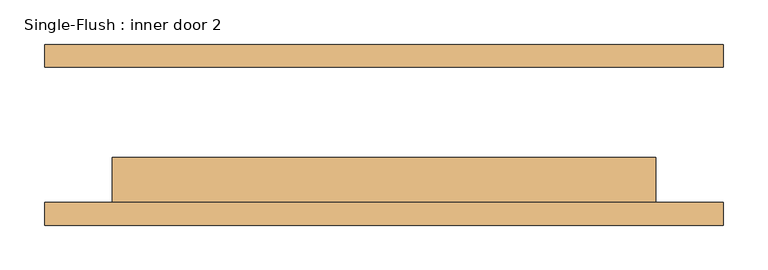
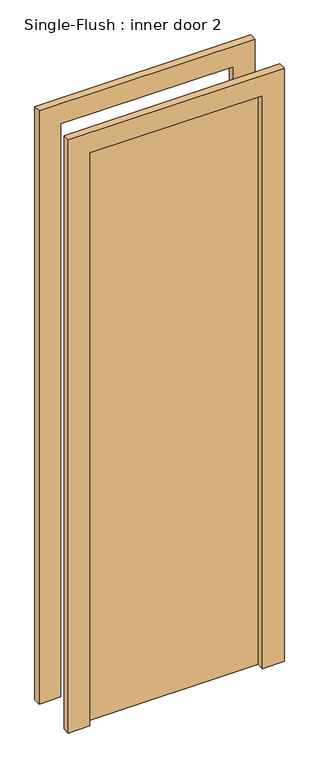
"""IFC4 building model written with IfcOpenShell, lengths in millimetres: door geometry, Single-Flush : inner door 2."""

from ifc_helpers import new_model, si_unit, frame, origin, origin_with_axes, place, context, project, spatial, polyline, outline, extrude, source, transform, mapped, element, save


def single_flush_inner_door_2_5ca4d175(model_context):
    return source(origin(), model_context, "Body", "SweptSolid", [
        extrude(outline(polyline([(2209.8, -381.0), (0.0, -381.0), (0.0, -304.8), (2133.6, -304.8), (2133.6, 304.8), (0.0, 304.8), (0.0, 381.0), (2209.8, 381.0), (2209.8, -381.0)])), frame((0.0, -101.6, 0.0), z_axis=(0.0, 1.0, 0.0), x_axis=(0.0, 0.0, 1.0)), (0.0, 0.0, 1.0), 25.4),
        extrude(outline(polyline([(2209.8, 381.0), (2209.8, -381.0), (0.0, -381.0), (0.0, -304.8), (2133.6, -304.8), (2133.6, 304.8), (0.0, 304.8), (0.0, 381.0), (2209.8, 381.0)])), frame((0.0, 76.2, 0.0), z_axis=(0.0, 1.0, 0.0), x_axis=(0.0, 0.0, 1.0)), (0.0, 0.0, 1.0), 25.4),
        extrude(outline(polyline([(304.8, -25.4), (304.8, -76.2), (-304.8, -76.2), (-304.8, -25.4), (304.8, -25.4)])), origin_with_axes(), (0.0, 0.0, 1.0), 2133.6),
    ])


if __name__ == "__main__":
    model = new_model("IFC4")
    model_context = context("Model", 3, world=origin())
    ifc_project = project(units=[si_unit("LENGTHUNIT", "METRE", prefix="MILLI")], contexts=[model_context])
    site = spatial("IfcSite", under=ifc_project)
    building = spatial("IfcBuilding", under=site)
    placement = place(None, origin())
    single_flush_inner_door_2_shape = single_flush_inner_door_2_5ca4d175(model_context)
    element("IfcDoor", 1, ObjectType="Single-Flush : inner door 2", at=placement, inside=building, context=model_context, shape_type="MappedRepresentation", body=[
        mapped(single_flush_inner_door_2_shape, transform((0.0, 0.0, 0.0), x_axis=(1.0, 0.0, 0.0), y_axis=(0.0, 1.0, 0.0), z_axis=(0.0, 0.0, 1.0))),
    ])
    save(model, "model.ifc")

# Revit data of these elements
# Type "Single-Flush : inner door 2"
#   Type Mark = "8"
#   Construction Type Id = "MDOOR"
#   Assembly Code = "C1020"
#   Analytic Construction = "Metal"
#   Thickness = 0' - 2"
#   Heat Transfer Coefficient (U) = 0.651978 BTU/(h·ft²·°F)
#   Height = 7' - 0"
#   Trim Projection Ext = 0' - 1"
#   Trim Projection Int = 0' - 1"
#   Trim Width = 0' - 3"
#   Width = 2' - 0"
#   Define Thermal Properties by = 1
#   Door Material = Door - Panel
#   Frame Material = Door - Frame
#   Visual Light Transmittance = 0
#   Solar Heat Gain Coefficient = 0
#   Function = (empty or 0)
#   Wall Closure = (empty or 0)
# Element 1 (IfcDoor, "Single-Flush : inner door 2")
#   Materials on its faces: "Door - Frame", "Door - Panel"
# Materials
#   "Door - Panel": class "Wood", colour RGB 210 159 95, transparency 0
#   "Door - Frame": colour RGB 118 70 51, transparency 0
